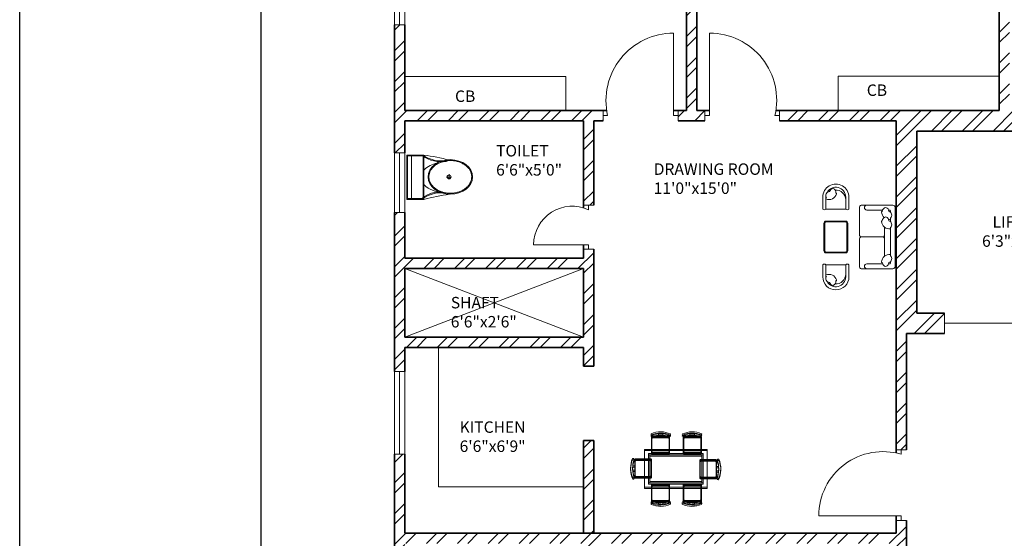
# Model space of a CAD drawing. Units: inches. Extents: x 2168 to 3056, y 1130 to 2629.
# Tile 21 of 42: x 2168 to 2598, y 2079 to 2305. Entities that reach past the tile are written whole.
import ezdxf

# ---------------------------------------------------------------- set-up
doc = ezdxf.new("R2010")
doc.units = ezdxf.units.IN
for name, color, linetype, lineweight in [('A-ANNO-DIMS', 2, 'Continuous', 18), ('A-ANNO-TEXT', 7, 'Continuous', 18), ('A-ANNO-TTLB', 7, 'Continuous', 25), ('A-AREA-IDEN', 7, 'Continuous', 18), ('A-DOOR', 21, 'Continuous', 18), ('A-EQPM-ELEV', 7, 'Continuous', 18), ('A-FLOR-CASE', 71, 'Continuous', 18), ('A-FLOR-FIXT', 9, 'Continuous', 18), ('A-FLOR-OTLN', 7, 'Continuous', 18), ('A-FURN', 8, 'Continuous', 13), ('A-GLAZ', 201, 'Continuous', 18), ('A-WALL', 7, 'Continuous', 35)]:
    doc.layers.add(name, color=color, linetype=linetype, lineweight=lineweight)
doc.layers.add('A-WALL-PATT', color=143, linetype='Continuous', lineweight=13, true_color=0x7aafdf)
doc.styles.get("Standard").update_dxf_attribs({"font": 'arial.ttf'})
doc.dimstyles.get("Standard").update_dxf_attribs({"dimtxt": 0.18, "dimasz": 0.18, "dimexe": 0.18, "dimexo": 0.0625, "dimgap": 0.09, "dimtad": 0, "dimtih": 1, "dimtoh": 1, "dimdec": 4, "dimzin": 0, "dimdsep": 46, "dimtxsty": 'Standard', "dimcen": 0.09, "dimadec": 0, "dimazin": 0, "dimtfac": 1, "dimtdec": 4, "dimtofl": 0, "dimtmove": 0, "dimatfit": 3, "dimfxl": 1, "dimtolj": 1, "dimtzin": 0, "dimarcsym": 0})

# ---------------------------------------------------------------- blocks, each defined once
blk = doc.blocks.new('A$C31115884')
for p, q in [((283, 498), (223, 498)), ((258, 466), (258, 523)), ((0, 200), (0, 0)), ((520, 200), (0, 200)), ((10, 190), (10, 10)), ((510, 190), (10, 190)), ((510, 10), (510, 190)), ((520, 0), (520, 200)), ((510, 54), (0, 54)), ((10, 10), (510, 10)), ((0, 0), (520, 0))]:
    blk.add_line(p, q)
blk.add_circle((256, 496), 23.6)
for centre, radius, start, end in [((2778, -205), 2807, 165.4549, 171.7133), ((-295, 403), 365, 324.2091, 9.3499), ((-295, 403), 375, 324.2091, 9.3499), ((806, 403), 365, 170.6501, 215.7909), ((3237, 905), 2807, 188.2867, 194.5451), ((384, 406), 293, 190.2774, 224.1564), ((139, 406), 293, 315.8436, 2.6563), ((806, 403), 375, 179.2036, 215.7909)]:
    blk.add_arc(centre, radius, start, end)
blk.add_ellipse((256, 510), major_axis=(0, -261), ratio=0.772727)
blk.add_open_spline([(256, 259), (263, 259), (270, 260), (288, 262), (299, 265), (320, 273), (330, 278), (350, 291), (360, 299), (378, 316), (386, 326), (402, 347), (409, 358), (421, 383), (427, 395), (436, 422), (440, 436), (445, 465), (447, 480), (448, 509), (448, 524), (445, 553), (443, 568), (436, 596), (432, 610), (422, 636), (416, 649), (402, 672), (395, 683), (379, 703), (370, 712), (351, 728), (341, 735), (321, 746), (310, 751), (289, 757), (278, 759), (256, 761), (245, 761), (223, 757), (212, 754), (191, 746), (181, 741), (161, 728), (151, 720), (133, 703), (125, 693), (110, 672), (103, 660), (90, 636), (85, 623), (76, 596), (72, 582), (67, 553), (66, 538), (64, 509), (65, 494), (68, 465), (70, 450), (77, 422), (81, 408), (91, 382), (97, 370), (111, 346), (118, 335), (135, 316), (144, 307), (162, 291), (172, 284), (193, 273), (203, 269), (225, 262), (236, 260), (250, 259), (253, 259), (256, 259)], degree=3, knots=[0, 0, 0, 0, 0.110105, 0.110105, 0.285049, 0.285049, 0.459994, 0.459994, 0.634938, 0.634938, 0.809882, 0.809882, 0.984827, 0.984827, 1.159771, 1.159771, 1.334715, 1.334715, 1.50966, 1.50966, 1.684604, 1.684604, 1.859549, 1.859549, 2.034493, 2.034493, 2.209437, 2.209437, 2.384382, 2.384382, 2.559326, 2.559326, 2.73427, 2.73427, 2.909215, 2.909215, 3.084159, 3.084159, 3.259103, 3.259103, 3.434048, 3.434048, 3.608992, 3.608992, 3.783936, 3.783936, 3.958881, 3.958881, 4.133825, 4.133825, 4.30877, 4.30877, 4.483714, 4.483714, 4.658658, 4.658658, 4.833603, 4.833603, 5.008547, 5.008547, 5.183491, 5.183491, 5.358436, 5.358436, 5.53338, 5.53338, 5.708324, 5.708324, 5.883269, 5.883269, 6.058213, 6.058213, 6.233158, 6.233158, 6.283185, 6.283185, 6.283185, 6.283185])
blk = doc.blocks.new('A$C1352')
at = {"color": 0}
for points in [[(0.003, 0.053), (0.003, 0.553, -0.414214), (0.053, 0.603), (0.753, 0.603, -0.414214), (0.803, 0.553), (0.803, 0.053, -0.414214), (0.753, 0.003), (0.053, 0.003, -0.414214)], [(0.023, 0.053), (0.023, 0.553, -0.414214), (0.053, 0.583), (0.753, 0.583, -0.414214), (0.783, 0.553), (0.783, 0.053, -0.414214), (0.753, 0.023), (0.053, 0.023, -0.414214)]]:
    blk.add_lwpolyline(points, format="xyb", close=True, dxfattribs=at)
blk = doc.blocks.new('CHAIR-LOUNGE')
blk.add_line((10.04, 5.71), (10.04, 10.98))
at = {"ltscale": 0.03}
blk.add_lwpolyline([(10.04, 10.98, -0.369229), (11.42, 10.98), (11.42, 5.7, -1), (0, 5.72), (0, 10.99, -0.369229), (1.39, 10.99)], format="xyb", close=True, dxfattribs=at)
blk.add_lwpolyline([(9.55, 3.71, -0.785087), (1.38, 5.71), (1.39, 10.99)], format="xyb")
for centre, radius, start, end in [((5.71, 6.93), 4.33, 179.9461, 273.658), ((5.63, 4.23), 0.207, 150.6238, 293.7423), ((8.67, 3.43), 3.35, 67.0143, 164.2857), ((8.41, 5.02), 1.73, 272.9922, 34.1401), ((5.71, 5.71), 4.33, 358.8536, 359.9461), ((7.44, 3.63), 1.78, 166.6403, 249.4695), ((6.65, 3.91), 1.95, 274.9999, 341.3534)]:
    blk.add_arc(centre, radius, start, end)
blk = doc.blocks.new('TABLE-DINING')
for points in [[(0, 17.02), (27.45, 17.02), (27.45, 0.55), (0, 0.55)], [(0, 17.02), (27.45, 17.02), (27.45, 0.55), (0, 0.55)], [(0, 16.47), (27.45, 16.47), (27.45, 0), (0, 0)], [(0, 16.47), (27.45, 16.47), (27.45, 0), (0, 0)], [(1.83, 15.19), (25.62, 15.19), (25.62, 2.38), (1.83, 2.38)], [(1.83, 15.19), (25.62, 15.19), (25.62, 2.38), (1.83, 2.38)], [(1.83, 14.64), (25.62, 14.64), (25.62, 1.83), (1.83, 1.83)], [(1.83, 14.64), (25.62, 14.64), (25.62, 1.83), (1.83, 1.83)], [(2.38, 14.64), (25.07, 14.64), (25.07, 2.93), (2.38, 2.93)], [(2.38, 14.64), (25.07, 14.64), (25.07, 2.93), (2.38, 2.93)], [(2.38, 14.09), (25.07, 14.09), (25.07, 2.38), (2.38, 2.38)], [(2.38, 14.09), (25.07, 14.09), (25.07, 2.38), (2.38, 2.38)]]:
    blk.add_lwpolyline(points, close=True)
blk = doc.blocks.new('CUPBOARD-BEDROOM')
blk.add_lwpolyline([(0, 14.89), (70.36, 14.89), (70.36, 0), (0, 0)], close=True)
blk = doc.blocks.new('CHAIR-DINING-SIDE')
for points in [[(7.85, 2.38, 0.414214), (8.33, 2.86), (8.33, 9.24, 0.414214), (7.85, 9.73), (0.91, 9.73, 0.414214), (0.42, 9.24), (0.42, 2.86, 0.414214), (0.91, 2.38), (7.85, 2.38)], [(7.85, 2.38, 0.414214), (8.33, 2.86), (8.33, 9.24, 0.414214), (7.85, 9.73), (0.91, 9.73, 0.414214), (0.42, 9.24), (0.42, 2.86, 0.414214), (0.91, 2.38), (7.85, 2.38)], [(7.85, 1.83, 0.414214), (8.33, 2.31), (8.33, 8.69, 0.414214), (7.85, 9.18), (0.91, 9.18, 0.414214), (0.42, 8.69), (0.42, 2.31, 0.414214), (0.91, 1.83), (7.85, 1.83)], [(7.85, 1.83, 0.414214), (8.33, 2.31), (8.33, 8.69, 0.414214), (7.85, 9.18), (0.91, 9.18, 0.414214), (0.42, 8.69), (0.42, 2.31, 0.414214), (0.91, 1.83), (7.85, 1.83)], [(8.06, 2.08, -0.175809), (0.59, 2.13, 0.578392), (0.02, 1.51, 0.214524), (8.46, 1.4, 0.552014), (8.06, 2.08, -0.065079)], [(8.06, 2.08, -0.175809), (0.59, 2.13, 0.578392), (0.02, 1.51, 0.214524), (8.46, 1.4, 0.552014), (8.06, 2.08, -0.065079)], [(8.06, 1.53, -0.175809), (0.59, 1.58, 0.578392), (0.02, 0.96, 0.214524), (8.46, 0.85, 0.552014), (8.06, 1.53, -0.065079)], [(8.06, 1.53, -0.175809), (0.59, 1.58, 0.578392), (0.02, 0.96, 0.214524), (8.46, 0.85, 0.552014), (8.06, 1.53, -0.065079)], [(3.34, 2.38), (3.34, 1.5, -0.064759)], [(3.34, 2.38), (3.34, 1.5, -0.064759)], [(3.34, 1.83), (3.34, 0.95, -0.064759)], [(3.34, 1.83), (3.34, 0.95, -0.064759)]]:
    blk.add_lwpolyline(points, format="xyb")
for points in [[(7.84, 2.6), (1.13, 2.6, -0.414214), (0.64, 3.08), (0.64, 9.02, -0.414214), (1.13, 9.51), (7.84, 9.51, -0.512069), (8.11, 9.02), (8.11, 3.08, -0.512069)], [(7.84, 2.6), (1.13, 2.6, -0.414214), (0.64, 3.08), (0.64, 9.02, -0.414214), (1.13, 9.51), (7.84, 9.51, -0.512069), (8.11, 9.02), (8.11, 3.08, -0.512069)], [(7.84, 2.05), (1.13, 2.05, -0.414214), (0.64, 2.53), (0.64, 8.48, -0.414214), (1.13, 8.96), (7.84, 8.96, -0.512069), (8.11, 8.48), (8.11, 2.53, -0.512069)], [(7.84, 2.05), (1.13, 2.05, -0.414214), (0.64, 2.53), (0.64, 8.48, -0.414214), (1.13, 8.96), (7.84, 8.96, -0.512069), (8.11, 8.48), (8.11, 2.53, -0.512069)]]:
    blk.add_lwpolyline(points, format="xyb", close=True)
for points in [[(5.29, 1.48), (5.29, 2.38)], [(5.29, 1.48), (5.29, 2.38)], [(5.29, 0.93), (5.29, 1.83)], [(5.29, 0.93), (5.29, 1.83)]]:
    blk.add_lwpolyline(points)
blk = doc.blocks.new('WIN-60-OPPOSED-JAMBS')
for p, q in [((2.25, 60), (0, 60)), ((0, 60), (4.5, 60)), ((0, 60), (0, 0)), ((2.25, 0), (2.25, 60)), ((4.5, 60), (4.5, 0)), ((0, 0), (4.5, 0)), ((4.5, 0), (2.25, 0))]:
    blk.add_line(p, q)
blk = doc.blocks.new('WIN-36')
for p, q in [((2.25, 36), (0, 36)), ((0, 36), (4.5, 36)), ((0, 36), (0, 0)), ((2.25, 0), (2.25, 36)), ((4.5, 36), (4.5, 0)), ((0, 0), (4.5, 0)), ((4.5, 0), (2.25, 0))]:
    blk.add_line(p, q)
blk = doc.blocks.new('*D41')
at = {"layer": 'A-ANNO-DIMS', "color": 0, "lineweight": -2, "transparency": 16777216}
for p, q in [((2331.73, 2478.39), (2273.32, 2478.39)), ((2273.5, 2478.21), (2273.5, 1928.07)), ((2273.5, 1377.57), (2273.5, 1927.71)), ((2331.73, 1377.39), (2273.32, 1377.39))]:
    blk.add_line(p, q, dxfattribs=at)
at = {"layer": 'A-ANNO-DIMS', "color": 0, "transparency": 16777216}
for points in [[(2273.47, 2478.21), (2273.53, 2478.21), (2273.5, 2478.39)], [(2273.47, 1377.57), (2273.53, 1377.57), (2273.5, 1377.39)]]:
    blk.add_solid(points, dxfattribs=at)
at = {"layer": 'Defpoints', "color": 0, "transparency": 16777216}
for p in [(2273.5, 2478.39), (2331.8, 2478.39), (2331.8, 1377.39)]:
    blk.add_point(p, dxfattribs=at)
at = {"layer": 'A-ANNO-DIMS', "color": 0, "transparency": 16777216, "insert": (2273.5, 1927.89), "char_height": 0.18, "attachment_point": 5}
blk.add_mtext('\\A1;1101', dxfattribs=at)

msp = doc.modelspace()

# ---------------------------------------------------------------- hatches: boundary and pattern name
at = {"layer": 'A-WALL-PATT'}
h = msp.add_hatch(dxfattribs=at)
h.set_pattern_fill('ANSI32', color=256)
h.paths.add_polyline_path([(2463.8, 2409.39), (2467.39, 2409.39), (2467.39, 2413.89), (2454.77, 2413.89), (2454.77, 2411.64), (2454.77, 2409.39), (2459.3, 2409.39), (2459.3, 2265.39), (2455.64, 2265.39), (2455.64, 2260.89), (2467.35, 2260.89), (2467.35, 2263.14), (2467.35, 2265.39), (2463.8, 2265.39)])
h.paths.add_polyline_path([(2431.6, 2413.89), (2409.65, 2413.89), (2409.65, 2409.39), (2431.6, 2409.39), (2431.6, 2411.64)])
h.paths.add_polyline_path([(2349.65, 2413.89), (2331.8, 2413.89), (2331.8, 2362.67), (2336.3, 2362.67), (2336.3, 2409.39), (2349.65, 2409.39), (2349.65, 2411.64)])
h.paths.add_polyline_path([(2634.15, 2411.64), (2634.15, 2413.89), (2562.29, 2413.89), (2562.29, 2409.39), (2595.8, 2409.39), (2595.8, 2280.31), (2595.83, 2280.31), (2595.83, 2265.39), (2499.91, 2265.39), (2499.91, 2260.89), (2550.8, 2260.89), (2550.8, 2117.31), (2555.3, 2117.31), (2555.3, 2168.08), (2571.93, 2168.08), (2571.93, 2176.89), (2559.8, 2176.89), (2559.8, 2256.39), (2640.8, 2256.39), (2640.8, 2176.89), (2626.43, 2176.89), (2626.43, 2168.08), (2645.3, 2168.08), (2645.3, 2116.64), (2649.8, 2116.64), (2649.8, 2260.89), (2691.25, 2260.89), (2691.25, 2263.14), (2691.25, 2265.39), (2670.65, 2265.39), (2670.65, 2265.36), (2600.3, 2265.36), (2600.3, 2280.26), (2600.3, 2409.39), (2634.15, 2409.39)])
h.paths.add_polyline_path([(2600.3, 2473.89), (2612.84, 2473.89), (2612.84, 2478.39), (2572.64, 2478.39), (2572.64, 2473.89), (2595.8, 2473.89), (2595.8, 2413.89), (2600.3, 2413.89)])
h.paths.add_polyline_path([(2535.8, 2473.89), (2548.64, 2473.89), (2548.64, 2478.39), (2531.4, 2478.39), (2531.4, 2413.89), (2521.6, 2413.89), (2521.6, 2409.39), (2539.24, 2409.39), (2539.24, 2411.64), (2539.24, 2413.89), (2535.8, 2413.89)])
h.paths.add_polyline_path([(2664.8, 2478.39), (2636.84, 2478.39), (2636.84, 2473.89), (2660.3, 2473.89), (2660.3, 2413.89), (2656.17, 2413.89), (2656.17, 2409.39), (2671.68, 2409.39), (2671.68, 2411.64), (2671.68, 2413.89), (2664.8, 2413.89)])
h.paths.add_polyline_path([(2705.94, 2413.89), (2695.68, 2413.89), (2695.68, 2409.39), (2705.94, 2409.39)])
h.paths.add_polyline_path([(2741.35, 2413.89), (2728.73, 2413.89), (2728.73, 2411.64), (2728.73, 2409.39), (2732.3, 2409.39), (2732.3, 2265.39), (2725.73, 2265.39), (2725.73, 2260.89), (2740.92, 2260.89), (2740.92, 2263.14), (2740.92, 2265.39), (2736.8, 2265.39), (2736.8, 2409.39), (2741.35, 2409.39)])
h.paths.add_polyline_path([(2785.65, 2413.89), (2764.55, 2413.89), (2764.49, 2409.39), (2785.65, 2409.39), (2785.65, 2411.64)])
h.paths.add_polyline_path([(2864.3, 2413.89), (2845.65, 2413.89), (2845.65, 2409.39), (2859.8, 2409.39), (2859.8, 2368.43), (2864.3, 2368.43)])
h.paths.add_polyline_path([(2864.3, 2308.43), (2862.05, 2308.43), (2859.8, 2308.43), (2859.8, 2265.39), (2774.48, 2265.39), (2774.48, 2263.14), (2774.48, 2260.89), (2781.8, 2260.89), (2781.8, 2226.65), (2786.3, 2226.65), (2786.3, 2260.89), (2859.8, 2260.89), (2859.8, 2241.35), (2864.3, 2241.35)])
h.paths.add_polyline_path([(2864.3, 2217.35), (2862.05, 2217.35), (2859.8, 2217.35), (2859.8, 2200.89), (2786.3, 2200.89), (2786.3, 2205.93), (2784.05, 2205.93), (2781.8, 2205.93), (2781.8, 2150.97), (2786.3, 2150.97), (2786.3, 2161.89), (2859.8, 2161.89), (2859.8, 2144.42), (2864.3, 2144.42)])
h.paths.add_polyline_path([(2859.8, 2196.39), (2859.8, 2166.39), (2786.3, 2166.39), (2786.3, 2196.39)], flags=16)
h.paths.add_polyline_path([(2864.3, 2108.42), (2862.05, 2108.42), (2859.8, 2108.42), (2859.8, 2080.89), (2786.3, 2080.89), (2786.3, 2111.99), (2781.8, 2111.99), (2781.8, 2080.89), (2649.8, 2080.89), (2649.8, 2086.04), (2647.55, 2086.04), (2645.3, 2086.04), (2645.3, 2071.74), (2649.8, 2071.74), (2649.8, 2076.39), (2781.8, 2076.39), (2781.8, 2041.79), (2786.3, 2041.79), (2786.3, 2076.39), (2859.8, 2076.39), (2859.8, 2058.58), (2864.3, 2058.58)])
h.paths.add_polyline_path([(2864.3, 2022.58), (2859.8, 2022.58), (2859.8, 1992.39), (2786.3, 1992.39), (2786.3, 1999.57), (2781.8, 1999.57), (2781.8, 1848.09), (2784.05, 1848.09), (2786.3, 1848.09), (2786.3, 1851.39), (2859.8, 1851.39), (2859.8, 1838.26), (2864.3, 1838.26)], flags=17)
h.paths.add_polyline_path([(2859.8, 1987.89), (2859.8, 1855.89), (2786.3, 1855.89), (2786.3, 1987.89)], flags=16)
h.paths.add_polyline_path([(2823.05, 1987.89), (2841.42, 1921.89), (2823.05, 1855.89)], flags=0)
h.paths.add_polyline_path([(2864.3, 1814.26), (2859.8, 1814.26), (2859.8, 1791.39), (2786.3, 1791.39), (2786.3, 1825.66), (2784.05, 1825.66), (2781.8, 1825.66), (2781.8, 1791.39), (2720.15, 1791.39), (2720.15, 1791.27), (2649.8, 1791.27), (2649.8, 1806.16), (2649.8, 2038.98), (2647.55, 2038.98), (2645.3, 2038.98), (2645.3, 1783.93), (2649.8, 1783.93), (2649.8, 1786.89), (2781.8, 1786.89), (2781.8, 1746.79), (2786.3, 1746.79), (2786.3, 1786.89), (2859.8, 1786.89), (2859.8, 1770.08), (2864.3, 1770.08)])
h.paths.add_polyline_path([(2864.3, 1734.08), (2862.05, 1734.08), (2859.8, 1734.08), (2859.8, 1705.89), (2786.3, 1705.89), (2786.3, 1714.17), (2781.8, 1714.17), (2781.8, 1660.53), (2786.3, 1660.53), (2786.3, 1666.89), (2859.8, 1666.89), (2859.8, 1648.34), (2864.3, 1648.34)])
h.paths.add_polyline_path([(2786.3, 1701.39), (2859.8, 1701.39), (2859.8, 1671.39), (2786.3, 1671.39)], flags=16)
h.paths.add_polyline_path([(2649.8, 1756.58), (2647.55, 1756.58), (2645.3, 1756.58), (2645.3, 1606.89), (2555.3, 1606.89), (2555.3, 1749.51), (2553.05, 1749.51), (2550.8, 1749.51), (2550.8, 1606.89), (2503.01, 1606.89), (2503.01, 1604.64), (2503.01, 1602.39), (2595.8, 1602.39), (2595.85, 1602.39), (2595.85, 1587.5), (2595.8, 1458.39), (2561.5, 1458.39), (2561.5, 1456.14), (2561.5, 1453.89), (2595.8, 1453.89), (2595.8, 1381.89), (2573.44, 1381.89), (2573.44, 1377.39), (2613.01, 1377.39), (2613.01, 1379.64), (2613.01, 1381.89), (2600.3, 1381.89), (2600.3, 1453.89), (2634.33, 1453.89), (2634.33, 1458.39), (2600.3, 1458.39), (2600.3, 1602.39), (2670.65, 1602.39), (2694.09, 1602.39), (2694.09, 1606.89), (2649.8, 1606.89)])
h.paths.add_polyline_path([(2736.8, 1602.39), (2741.56, 1602.39), (2741.56, 1606.89), (2726.2, 1606.89), (2726.2, 1604.64), (2726.2, 1602.39), (2732.3, 1602.39), (2732.3, 1458.39), (2727.9, 1458.39), (2727.9, 1453.89), (2740.82, 1453.89), (2740.82, 1456.14), (2740.82, 1458.39), (2736.8, 1458.39)])
h.paths.add_polyline_path([(2859.8, 1606.89), (2786.3, 1606.89), (2786.3, 1637.33), (2784.05, 1637.33), (2781.8, 1637.33), (2781.8, 1606.89), (2775.61, 1606.89), (2775.61, 1602.39), (2859.8, 1602.39)])
h.paths.add_polyline_path([(2864.3, 1624.34), (2862.05, 1624.34), (2859.8, 1624.34), (2859.8, 1570.39), (2864.3, 1570.39)])
h.paths.add_polyline_path([(2864.3, 1510.39), (2862.05, 1510.39), (2859.8, 1510.39), (2859.8, 1458.39), (2846.73, 1458.39), (2846.73, 1456.14), (2846.73, 1453.89), (2864.3, 1453.89)])
h.paths.add_polyline_path([(2786.73, 1458.39), (2765.44, 1458.39), (2765.44, 1453.89), (2786.73, 1453.89)])
h.paths.add_polyline_path([(2706, 1458.39), (2695.36, 1458.39), (2695.36, 1453.89), (2706, 1453.89), (2706, 1456.14)])
h.paths.add_polyline_path([(2671.36, 1456.14), (2671.36, 1458.39), (2655.99, 1458.39), (2655.99, 1456.14), (2655.99, 1453.89), (2660.3, 1453.89), (2660.3, 1381.89), (2637.01, 1381.89), (2637.01, 1377.39), (2664.8, 1377.39), (2664.8, 1453.89), (2671.36, 1453.89)], flags=17)
h.paths.add_polyline_path([(2539.83, 1458.39), (2520.24, 1458.39), (2520.24, 1453.89), (2531.3, 1453.89), (2531.3, 1377.39), (2546.45, 1377.39), (2546.45, 1379.64), (2546.45, 1381.89), (2535.8, 1381.89), (2535.8, 1453.89), (2539.83, 1453.89)], flags=17)
h.paths.add_polyline_path([(2496.24, 1458.39), (2489.13, 1458.39), (2489.13, 1453.89), (2496.24, 1453.89), (2496.24, 1456.14)])
h.paths.add_polyline_path([(2467.43, 1456.14), (2467.43, 1458.39), (2463.8, 1458.39), (2463.8, 1602.39), (2468.24, 1602.39), (2468.24, 1605.7), (2468.24, 1606.89), (2454.6, 1606.89), (2454.6, 1602.39), (2459.3, 1602.39), (2459.3, 1458.39), (2454.24, 1458.39), (2454.24, 1453.89), (2467.43, 1453.89)])
h.paths.add_polyline_path([(2431.6, 1456.14), (2431.6, 1458.39), (2411.39, 1458.39), (2411.39, 1453.89), (2431.6, 1453.89)])
h.paths.add_polyline_path([(2351.39, 1458.39), (2336.3, 1458.39), (2336.3, 1490.69), (2334.05, 1490.69), (2331.8, 1490.69), (2331.8, 1453.89), (2351.39, 1453.89), (2351.39, 1456.14)])
h.paths.add_polyline_path([(2336.3, 1629.7), (2331.8, 1629.7), (2331.8, 1552.32), (2336.3, 1552.32), (2336.3, 1602.39), (2406.65, 1602.39), (2423.47, 1602.39), (2423.47, 1606.89), (2418.8, 1606.89), (2418.8, 1643.68), (2416.55, 1643.68), (2414.3, 1643.68), (2414.3, 1606.89), (2336.3, 1606.89)])
h.paths.add_polyline_path([(2418.8, 1714.38), (2414.3, 1714.38), (2414.3, 1705.89), (2336.3, 1705.89), (2336.3, 1731.32), (2334.05, 1731.32), (2331.8, 1731.32), (2331.8, 1653.7), (2334.05, 1653.7), (2336.3, 1653.7), (2336.3, 1666.89), (2414.3, 1666.89), (2414.3, 1663.59), (2418.8, 1663.59)])
h.paths.add_polyline_path([(2336.3, 1701.39), (2414.3, 1701.39), (2414.3, 1671.39), (2336.3, 1671.39)], flags=16)
h.paths.add_polyline_path([(2555.3, 2040.06), (2550.8, 2040.06), (2550.8, 1791.39), (2550.56, 1791.2), (2480.2, 1791.2), (2418.8, 1791.39), (2418.8, 1825.45), (2416.55, 1825.45), (2414.3, 1825.45), (2414.3, 1791.39), (2336.3, 1791.39), (2336.3, 1806.41), (2331.8, 1806.41), (2331.8, 1767.32), (2336.3, 1767.32), (2336.3, 1786.89), (2414.3, 1786.89), (2414.3, 1745.46), (2418.8, 1745.46), (2418.8, 1786.89), (2550.8, 1786.89), (2550.8, 1783.01), (2555.3, 1783.01)])
h.paths.add_polyline_path([(2418.8, 1923.39), (2423.21, 1923.39), (2423.21, 1925.64), (2423.21, 1927.89), (2418.8, 1927.89), (2418.8, 2000.05), (2414.3, 2000.05), (2414.3, 1992.39), (2336.3, 1992.39), (2336.3, 1987.89), (2414.3, 1987.89), (2414.3, 1855.89), (2336.3, 1855.89), (2336.3, 1851.39), (2414.3, 1851.39), (2414.3, 1846.76), (2418.8, 1846.76)], flags=17)
h.paths.add_polyline_path([(2336.3, 2019.29), (2334.05, 2019.29), (2331.8, 2019.29), (2331.8, 1830.41), (2336.3, 1830.41)], flags=17)
h.paths.add_polyline_path([(2550.8, 1927.89), (2453.54, 1927.89), (2453.54, 1925.64), (2453.54, 1923.39), (2550.8, 1923.39)], flags=17)
h.paths.add_polyline_path([(2744.99, 1927.89), (2649.8, 1927.89), (2649.8, 1923.39), (2744.99, 1923.39), (2744.99, 1925.64)], flags=17)
h.paths.add_polyline_path([(2555.3, 2086.46), (2553.05, 2086.46), (2550.8, 2086.46), (2550.8, 2080.89), (2418.8, 2080.89), (2336.3, 2080.89), (2336.3, 2115.4), (2334.05, 2115.4), (2331.8, 2115.4), (2331.8, 2055.29), (2336.3, 2055.29), (2336.3, 2076.39), (2550.8, 2076.39), (2550.8, 2071.54), (2555.3, 2071.54)])
h.paths.add_polyline_path([(2418.8, 2121.39), (2414.3, 2121.39), (2414.3, 2080.89), (2418.8, 2080.89)])
h.paths.add_polyline_path([(2418.8, 2076.39), (2414.3, 2076.39), (2414.3, 2035.12), (2418.8, 2035.12)])
h.paths.add_polyline_path([(2422.87, 2263.14), (2422.87, 2265.39), (2406.65, 2265.39), (2406.65, 2265.36), (2336.3, 2265.36), (2336.3, 2280.25), (2336.3, 2302.67), (2334.05, 2302.67), (2331.8, 2302.67), (2331.8, 2246.85), (2336.3, 2246.85), (2336.3, 2260.89), (2414.3, 2260.89), (2414.3, 2224), (2418.8, 2224), (2418.8, 2260.89), (2422.87, 2260.89)])
h.paths.add_polyline_path([(2418.8, 2204.78), (2416.55, 2204.78), (2414.3, 2204.78), (2414.3, 2200.89), (2336.3, 2200.89), (2336.3, 2220.85), (2331.8, 2220.85), (2331.8, 2151.4), (2336.3, 2151.4), (2336.3, 2161.89), (2414.3, 2161.89), (2414.3, 2153.73), (2418.8, 2153.73)])
h.paths.add_polyline_path([(2414.3, 2196.39), (2414.3, 2166.39), (2336.3, 2166.39), (2336.3, 2196.39)], flags=16)
h.paths.add_polyline_path([(2375.3, 2181.39), (2336.3, 2166.39), (2336.3, 2196.39)], flags=0)
h.paths.add_polyline_path([(2809.6, 2172.34), (2838.8, 2172.34), (2838.8, 2191), (2809.6, 2191)], flags=8)
h.paths.add_polyline_path([(2849.75, 1919.59), (2849.75, 1952.67), (2831.09, 1952.67), (2831.09, 1919.59)], flags=8)
h.paths.add_polyline_path([(2808.87, 1901.97), (2808.87, 1937.85), (2790.15, 1937.85), (2790.15, 1901.97)], flags=8)
h.paths.add_polyline_path([(2806.28, 1671.9), (2835.49, 1671.9), (2835.49, 1690.55), (2806.28, 1690.55)], flags=8)
h.paths.add_polyline_path([(2353.19, 1676.55), (2382.39, 1676.55), (2382.39, 1695.21), (2353.19, 1695.21)], flags=8)
h.paths.add_polyline_path([(2360.08, 1832.31), (2389.24, 1832.31), (2389.24, 1850.97), (2360.08, 1850.97)], flags=25)
h.paths.add_polyline_path([(2354.82, 2167.82), (2384.03, 2167.82), (2384.03, 2186.48), (2354.82, 2186.48)], flags=8)

# ---------------------------------------------------------------- linework, layer by layer
at = {"layer": 'A-ANNO-TTLB'}
msp.add_lwpolyline([(2168.16, 2629.19), (3055.63, 2629.19), (3055.63, 1130.19), (2168.16, 1130.19)], close=True, dxfattribs=at)
at = {"layer": 'A-DOOR'}
for p, q in [((2453.64, 2263.16), (2453.64, 2299.16)), ((2469.35, 2263.14), (2469.35, 2299.14)), ((2422.87, 2265.39), (2422.87, 2260.89)), ((2422.87, 2260.89), (2422.87, 2263.14)), ((2422.87, 2263.14), (2424.87, 2263.14)), ((2455.64, 2263.14), (2453.64, 2263.16)), ((2455.64, 2265.39), (2455.64, 2260.89)), ((2455.64, 2260.89), (2455.64, 2263.14)), ((2467.35, 2265.39), (2467.35, 2260.89)), ((2467.35, 2260.89), (2467.35, 2263.14)), ((2467.35, 2263.14), (2469.35, 2263.14)), ((2499.91, 2263.14), (2497.91, 2263.14)), ((2499.91, 2265.39), (2499.91, 2260.89)), ((2499.91, 2260.89), (2499.91, 2265.39)), ((2414.3, 2224), (2418.8, 2224)), ((2418.8, 2224), (2416.55, 2224)), ((2416.55, 2224), (2416.55, 2222)), ((2416.55, 2206.78), (2392.55, 2206.78)), ((2416.55, 2204.78), (2416.55, 2206.78)), ((2414.3, 2204.78), (2418.8, 2204.78)), ((2418.8, 2204.78), (2416.55, 2204.78)), ((2550.8, 2117.31), (2555.3, 2117.31)), ((2553.05, 2117.31), (2553.05, 2115.31)), ((2553.05, 2088.46), (2517.05, 2088.46)), ((2550.8, 2086.46), (2555.3, 2086.46)), ((2553.05, 2086.46), (2553.05, 2088.46)), ((2555.3, 2086.46), (2553.05, 2086.46))]:
    msp.add_line(p, q, dxfattribs=at)
for centre, radius, start, end in [((2453.64, 2269.65), 29.5, 90, 192.7563), ((2469.35, 2269.81), 29.33, 346.8551, 90), ((2409.37, 2206.78), 16.82, 64.7394, 180), ((2545.06, 2088.46), 28.01, 73.4344, 180)]:
    msp.add_arc(centre, radius, start, end, dxfattribs=at)
at = {"layer": 'A-EQPM-ELEV'}
for p, q in [((2571.93, 2176.89), (2571.93, 2168.08)), ((2626.43, 2172.48), (2571.93, 2172.48))]:
    msp.add_line(p, q, dxfattribs=at)
at = {"layer": 'A-FLOR-CASE'}
for p, q in [((2350.95, 2101.14), (2350.95, 2161.89)), ((2414.3, 2101.14), (2350.95, 2101.14))]:
    msp.add_line(p, q, dxfattribs=at)
at = {"layer": 'A-FLOR-OTLN'}
for p, q in [((2336.3, 2166.39), (2414.3, 2196.39)), ((2336.3, 2196.39), (2414.3, 2166.39)), ((2414.3, 2166.39), (2414.3, 2166.39))]:
    msp.add_line(p, q, dxfattribs=at)
at = {"layer": 'A-FURN'}
for p, q in [((2544.93, 2221.92), (2538, 2221.92)), ((2547.56, 2221.92), (2548.04, 2221.92)), ((2548.38, 2221.57), (2548.38, 2220.94)), ((2548.38, 2216.78), (2548.38, 2218.44)), ((2548.38, 2217.42), (2548.38, 2216.78)), ((2548.38, 2201.87), (2548.38, 2214.29)), ((2538, 2198.39), (2544.93, 2198.39)), ((2547.56, 2198.39), (2548.04, 2198.39)), ((2548.38, 2198.74), (2548.38, 2199.37))]:
    msp.add_line(p, q, dxfattribs=at)
at = {"layer": 'A-FURN', "ltscale": 0.03}
msp.add_lwpolyline([(2535.58, 2210.15, 0.414214), (2534.89, 2209.45), (2534.89, 2197.01, 0.414214), (2535.58, 2196.31), (2549.42, 2196.31, 0.414214), (2550.46, 2197.35), (2550.46, 2222.96, 0.414214), (2549.42, 2224), (2535.58, 2224, 0.414214), (2534.89, 2223.3), (2534.89, 2210.86, 0.414214), (2535.58, 2210.16)], format="xyb", dxfattribs=at)
at = {"layer": 'A-FURN'}
for points in [[(2545.7, 2214.42), (2545.7, 2211.02, -0.414214), (2544.84, 2210.16), (2535.75, 2210.16, -0.414214), (2534.89, 2211.02), (2534.89, 2223.13, -0.414214), (2535.75, 2224)], [(2545.7, 2202.32), (2545.7, 2209.29, 0.414214), (2544.84, 2210.16), (2535.75, 2210.16, 0.414214), (2534.89, 2209.29), (2534.89, 2197.18, 0.414214), (2535.75, 2196.31)], [(2444.28, 2123.6, -0.175809), (2451.76, 2123.55, 0.578392), (2452.32, 2124.17, 0.214524), (2443.89, 2124.28, 0.552014), (2444.28, 2123.6, -0.065079)], [(2444.28, 2123.6, -0.175809), (2451.76, 2123.55, 0.578392), (2452.32, 2124.17, 0.214524), (2443.89, 2124.28, 0.552014), (2444.28, 2123.6, -0.065079)], [(2444.28, 2123.05, -0.175809), (2451.76, 2123, 0.578392), (2452.32, 2123.62, 0.214524), (2443.89, 2123.73, 0.552014), (2444.28, 2123.05, -0.065079)], [(2444.28, 2123.05, -0.175809), (2451.76, 2123, 0.578392), (2452.32, 2123.62, 0.214524), (2443.89, 2123.73, 0.552014), (2444.28, 2123.05, -0.065079)], [(2449, 2123.3), (2449, 2124.18, -0.064759)], [(2449, 2123.3), (2449, 2124.18, -0.064759)], [(2458.05, 2123.55, -0.578392), (2457.49, 2124.17, -0.214524), (2465.92, 2124.28, -0.552014), (2465.53, 2123.6, 0.175809), (2458.05, 2123.55)], [(2458.05, 2123.55, -0.578392), (2457.49, 2124.17, -0.214524), (2465.92, 2124.28, -0.552014), (2465.53, 2123.6, 0.175809), (2458.05, 2123.55)], [(2458.05, 2123, -0.578392), (2457.49, 2123.62, -0.214524), (2465.92, 2123.73, -0.552014), (2465.53, 2123.05, 0.175809), (2458.05, 2123)], [(2458.05, 2123, -0.578392), (2457.49, 2123.62, -0.214524), (2465.92, 2123.73, -0.552014), (2465.53, 2123.05, 0.175809), (2458.05, 2123)], [(2460.81, 2123.3), (2460.81, 2124.18, 0.064759)], [(2460.81, 2123.3), (2460.81, 2124.18, 0.064759)], [(2451.44, 2123.3), (2444.5, 2123.3, 0.414214), (2444.02, 2122.82), (2444.02, 2116.44, 0.414214), (2444.5, 2115.95), (2451.44, 2115.95, 0.414214), (2451.93, 2116.44), (2451.93, 2122.82, 0.414214), (2451.44, 2123.3)], [(2451.44, 2123.3), (2444.5, 2123.3, 0.414214), (2444.02, 2122.82), (2444.02, 2116.44, 0.414214), (2444.5, 2115.95), (2451.44, 2115.95, 0.414214), (2451.93, 2116.44), (2451.93, 2122.82, 0.414214), (2451.44, 2123.3)], [(2451.44, 2122.75), (2444.5, 2122.75, 0.414214), (2444.02, 2122.27), (2444.02, 2115.89, 0.414214), (2444.5, 2115.4), (2451.44, 2115.4, 0.414214), (2451.93, 2115.89), (2451.93, 2122.27, 0.414214), (2451.44, 2122.75)], [(2451.44, 2122.75), (2444.5, 2122.75, 0.414214), (2444.02, 2122.27), (2444.02, 2115.89, 0.414214), (2444.5, 2115.4), (2451.44, 2115.4, 0.414214), (2451.93, 2115.89), (2451.93, 2122.27, 0.414214), (2451.44, 2122.75)], [(2449, 2122.75), (2449, 2123.63, -0.064759)], [(2449, 2122.75), (2449, 2123.63, -0.064759)], [(2465.31, 2123.3, -0.414214), (2465.79, 2122.82), (2465.79, 2116.44, -0.414214), (2465.31, 2115.95), (2458.37, 2115.95, -0.414214), (2457.88, 2116.44), (2457.88, 2122.82, -0.414214), (2458.37, 2123.3), (2465.31, 2123.3)], [(2465.31, 2123.3, -0.414214), (2465.79, 2122.82), (2465.79, 2116.44, -0.414214), (2465.31, 2115.95), (2458.37, 2115.95, -0.414214), (2457.88, 2116.44), (2457.88, 2122.82, -0.414214), (2458.37, 2123.3), (2465.31, 2123.3)], [(2465.31, 2122.75, -0.414214), (2465.79, 2122.27), (2465.79, 2115.89, -0.414214), (2465.31, 2115.4), (2458.37, 2115.4, -0.414214), (2457.88, 2115.89), (2457.88, 2122.27, -0.414214), (2458.37, 2122.75), (2465.31, 2122.75)], [(2465.31, 2122.75, -0.414214), (2465.79, 2122.27), (2465.79, 2115.89, -0.414214), (2465.31, 2115.4), (2458.37, 2115.4, -0.414214), (2457.88, 2115.89), (2457.88, 2122.27, -0.414214), (2458.37, 2122.75), (2465.31, 2122.75)], [(2460.81, 2122.75), (2460.81, 2123.63, 0.064759)], [(2460.81, 2122.75), (2460.81, 2123.63, 0.064759)], [(2436.46, 2105.55, -0.578392), (2435.84, 2104.98, -0.214524), (2435.73, 2113.42, -0.552014), (2436.41, 2113.03, 0.175809), (2436.46, 2105.55)], [(2436.46, 2105.55, -0.578392), (2435.84, 2104.98, -0.214524), (2435.73, 2113.42, -0.552014), (2436.41, 2113.03, 0.175809), (2436.46, 2105.55)], [(2436.46, 2105, -0.578392), (2435.84, 2104.44, -0.214524), (2435.73, 2112.87, -0.552014), (2436.41, 2112.48, 0.175809), (2436.46, 2105)], [(2436.46, 2105, -0.578392), (2435.84, 2104.44, -0.214524), (2435.73, 2112.87, -0.552014), (2436.41, 2112.48, 0.175809), (2436.46, 2105)], [(2436.71, 2112.81, -0.414214), (2437.19, 2113.29), (2443.57, 2113.29, -0.414214), (2444.06, 2112.81), (2444.06, 2105.87, -0.414214), (2443.57, 2105.38), (2437.19, 2105.38, -0.414214), (2436.71, 2105.87), (2436.71, 2112.81)], [(2436.71, 2112.81, -0.414214), (2437.19, 2113.29), (2443.57, 2113.29, -0.414214), (2444.06, 2112.81), (2444.06, 2105.87, -0.414214), (2443.57, 2105.38), (2437.19, 2105.38, -0.414214), (2436.71, 2105.87), (2436.71, 2112.81)], [(2436.71, 2112.26, -0.414214), (2437.19, 2112.75), (2443.57, 2112.75, -0.414214), (2444.06, 2112.26), (2444.06, 2105.32, -0.414214), (2443.57, 2104.83), (2437.19, 2104.83, -0.414214), (2436.71, 2105.32), (2436.71, 2112.26)], [(2436.71, 2112.26, -0.414214), (2437.19, 2112.74), (2443.57, 2112.74, -0.414214), (2444.06, 2112.26), (2444.06, 2105.32, -0.414214), (2443.57, 2104.83), (2437.19, 2104.83, -0.414214), (2436.71, 2105.32), (2436.71, 2112.26)], [(2472.44, 2112.57, 0.414214), (2471.96, 2113.06), (2465.58, 2113.06, 0.414214), (2465.09, 2112.57), (2465.09, 2105.63, 0.414214), (2465.58, 2105.15), (2471.96, 2105.15, 0.414214), (2472.44, 2105.63), (2472.44, 2112.57)], [(2472.44, 2112.57, 0.414214), (2471.96, 2113.06), (2465.58, 2113.06, 0.414214), (2465.09, 2112.57), (2465.09, 2105.63, 0.414214), (2465.58, 2105.14), (2471.96, 2105.14, 0.414214), (2472.44, 2105.63), (2472.44, 2112.57)], [(2472.44, 2112.02, 0.414214), (2471.96, 2112.51), (2465.58, 2112.51, 0.414214), (2465.09, 2112.02), (2465.09, 2105.08, 0.414214), (2465.58, 2104.6), (2471.96, 2104.6, 0.414214), (2472.44, 2105.08), (2472.44, 2112.02)], [(2472.44, 2112.02, 0.414214), (2471.96, 2112.51), (2465.58, 2112.51, 0.414214), (2465.09, 2112.02), (2465.09, 2105.08, 0.414214), (2465.58, 2104.6), (2471.96, 2104.6, 0.414214), (2472.44, 2105.08), (2472.44, 2112.02)], [(2472.74, 2112.79, -0.175809), (2472.69, 2105.31, 0.578392), (2473.31, 2104.75, 0.214524), (2473.42, 2113.19, 0.552014), (2472.74, 2112.79, -0.065079)], [(2472.74, 2112.79, -0.175809), (2472.69, 2105.31, 0.578392), (2473.31, 2104.75, 0.214524), (2473.42, 2113.19, 0.552014), (2472.74, 2112.79, -0.065079)], [(2472.74, 2112.24, -0.175809), (2472.69, 2104.76, 0.578392), (2473.31, 2104.2, 0.214524), (2473.42, 2112.64, 0.552014), (2472.74, 2112.24, -0.065079)], [(2472.74, 2112.24, -0.175809), (2472.69, 2104.76, 0.578392), (2473.31, 2104.2, 0.214524), (2473.42, 2112.64, 0.552014), (2472.74, 2112.24, -0.065079)], [(2436.71, 2108.31), (2435.83, 2108.31, 0.064759)], [(2436.71, 2108.31), (2435.83, 2108.31, 0.064759)], [(2436.71, 2107.76), (2435.83, 2107.76, 0.064759)], [(2436.71, 2107.76), (2435.83, 2107.76, 0.064759)], [(2472.44, 2108.07), (2473.32, 2108.07, -0.064759)], [(2472.44, 2108.07), (2473.32, 2108.07, -0.064759)], [(2472.44, 2107.52), (2473.32, 2107.52, -0.064759)], [(2472.44, 2107.52), (2473.32, 2107.52, -0.064759)], [(2451.44, 2094.94), (2444.5, 2094.94, -0.414214), (2444.02, 2095.42), (2444.02, 2101.8, -0.414214), (2444.5, 2102.29), (2451.44, 2102.29, -0.414214), (2451.93, 2101.8), (2451.93, 2095.42, -0.414214), (2451.44, 2094.94)], [(2451.44, 2094.94), (2444.5, 2094.94, -0.414214), (2444.02, 2095.42), (2444.02, 2101.8, -0.414214), (2444.5, 2102.29), (2451.44, 2102.29, -0.414214), (2451.93, 2101.8), (2451.93, 2095.42, -0.414214), (2451.44, 2094.94)], [(2451.44, 2094.39), (2444.5, 2094.39, -0.414214), (2444.02, 2094.87), (2444.02, 2101.26, -0.414214), (2444.5, 2101.74), (2451.44, 2101.74, -0.414214), (2451.93, 2101.26), (2451.93, 2094.87, -0.414214), (2451.44, 2094.39)], [(2451.44, 2094.39), (2444.5, 2094.39, -0.414214), (2444.02, 2094.87), (2444.02, 2101.26, -0.414214), (2444.5, 2101.74), (2451.44, 2101.74, -0.414214), (2451.93, 2101.26), (2451.93, 2094.87, -0.414214), (2451.44, 2094.39)], [(2451.76, 2094.69, -0.578392), (2452.32, 2094.07, -0.214524), (2443.89, 2093.96, -0.552014), (2444.28, 2094.64, 0.175809), (2451.76, 2094.69)], [(2451.76, 2094.69, -0.578392), (2452.32, 2094.07, -0.214524), (2443.89, 2093.96, -0.552014), (2444.28, 2094.64, 0.175809), (2451.76, 2094.69)], [(2451.76, 2094.15, -0.578392), (2452.32, 2093.52, -0.214524), (2443.89, 2093.41, -0.552014), (2444.28, 2094.09, 0.175809), (2451.76, 2094.15)], [(2451.76, 2094.14, -0.578392), (2452.32, 2093.52, -0.214524), (2443.89, 2093.41, -0.552014), (2444.28, 2094.09, 0.175809), (2451.76, 2094.14)], [(2449, 2094.94), (2449, 2094.06, 0.064759)], [(2449, 2094.94), (2449, 2094.06, 0.064759)], [(2449, 2094.39), (2449, 2093.51, 0.064759)], [(2449, 2094.39), (2449, 2093.51, 0.064759)]]:
    msp.add_lwpolyline(points, format="xyb", dxfattribs=at)
for points in [[(2545.7, 2214.42), (2545.7, 2201.73)], [(2447.06, 2124.2), (2447.06, 2123.3)], [(2447.06, 2124.2), (2447.06, 2123.3)], [(2462.75, 2124.2), (2462.75, 2123.3)], [(2462.75, 2124.2), (2462.75, 2123.3)], [(2447.06, 2123.65), (2447.06, 2122.75)], [(2447.06, 2123.65), (2447.06, 2122.75)], [(2462.75, 2123.65), (2462.75, 2122.75)], [(2462.75, 2123.65), (2462.75, 2122.75)], [(2435.81, 2110.25), (2436.71, 2110.25)], [(2435.81, 2110.25), (2436.71, 2110.25)], [(2435.81, 2109.7), (2436.71, 2109.7)], [(2435.81, 2109.7), (2436.71, 2109.7)], [(2473.34, 2110.01), (2472.44, 2110.01)], [(2473.34, 2110.01), (2472.44, 2110.01)], [(2473.34, 2109.46), (2472.44, 2109.46)], [(2473.34, 2109.46), (2472.44, 2109.46)], [(2447.06, 2094.04), (2447.06, 2094.94)], [(2447.06, 2094.04), (2447.06, 2094.94)], [(2447.06, 2093.5), (2447.06, 2094.39)], [(2447.06, 2093.49), (2447.06, 2094.39)]]:
    msp.add_lwpolyline(points, dxfattribs=at)
for points in [[(2444.5, 2123.08), (2451.22, 2123.08, -0.414214), (2451.71, 2122.6), (2451.71, 2116.66, -0.414214), (2451.22, 2116.17), (2444.5, 2116.17, -0.512069), (2444.23, 2116.66), (2444.23, 2122.6, -0.512069)], [(2444.5, 2123.08), (2451.22, 2123.08, -0.414214), (2451.71, 2122.6), (2451.71, 2116.66, -0.414214), (2451.22, 2116.17), (2444.5, 2116.17, -0.512069), (2444.23, 2116.66), (2444.23, 2122.6, -0.512069)], [(2444.5, 2122.54), (2451.22, 2122.54, -0.414214), (2451.71, 2122.05), (2451.71, 2116.11, -0.414214), (2451.22, 2115.62), (2444.5, 2115.62, -0.512069), (2444.23, 2116.11), (2444.23, 2122.05, -0.512069)], [(2444.5, 2122.54), (2451.22, 2122.54, -0.414214), (2451.71, 2122.05), (2451.71, 2116.11, -0.414214), (2451.22, 2115.62), (2444.5, 2115.62, -0.512069), (2444.23, 2116.11), (2444.23, 2122.05, -0.512069)], [(2465.31, 2123.08), (2458.59, 2123.08, 0.414214), (2458.1, 2122.6), (2458.1, 2116.66, 0.414214), (2458.59, 2116.17), (2465.31, 2116.17, 0.512069), (2465.58, 2116.66), (2465.58, 2122.6, 0.512069)], [(2465.31, 2123.08), (2458.59, 2123.08, 0.414214), (2458.1, 2122.6), (2458.1, 2116.66, 0.414214), (2458.59, 2116.17), (2465.31, 2116.17, 0.512069), (2465.58, 2116.66), (2465.58, 2122.6, 0.512069)], [(2465.31, 2122.54), (2458.59, 2122.54, 0.414214), (2458.1, 2122.05), (2458.1, 2116.11, 0.414214), (2458.59, 2115.62), (2465.31, 2115.62, 0.512069), (2465.58, 2116.11), (2465.58, 2122.05, 0.512069)], [(2465.31, 2122.54), (2458.59, 2122.54, 0.414214), (2458.1, 2122.05), (2458.1, 2116.11, 0.414214), (2458.59, 2115.62), (2465.31, 2115.62, 0.512069), (2465.58, 2116.11), (2465.58, 2122.05, 0.512069)], [(2436.92, 2112.81), (2436.92, 2106.09, 0.414214), (2437.41, 2105.6), (2443.35, 2105.6, 0.414214), (2443.84, 2106.09), (2443.84, 2112.81, 0.512069), (2443.35, 2113.08), (2437.41, 2113.08, 0.512069)], [(2436.92, 2112.81), (2436.92, 2106.09, 0.414214), (2437.41, 2105.6), (2443.35, 2105.6, 0.414214), (2443.84, 2106.09), (2443.84, 2112.81, 0.512069), (2443.35, 2113.07), (2437.41, 2113.07, 0.512069)], [(2436.92, 2112.26), (2436.92, 2105.54, 0.414214), (2437.41, 2105.05), (2443.35, 2105.05, 0.414214), (2443.84, 2105.54), (2443.84, 2112.26, 0.512069), (2443.35, 2112.53), (2437.41, 2112.53, 0.512069)], [(2436.92, 2112.26), (2436.92, 2105.54, 0.414214), (2437.41, 2105.05), (2443.35, 2105.05, 0.414214), (2443.84, 2105.54), (2443.84, 2112.26, 0.512069), (2443.35, 2112.53), (2437.41, 2112.53, 0.512069)], [(2472.22, 2112.57), (2472.22, 2105.85, -0.414214), (2471.74, 2105.36), (2465.79, 2105.36, -0.414214), (2465.31, 2105.85), (2465.31, 2112.57, -0.512069), (2465.79, 2112.84), (2471.74, 2112.84, -0.512069)], [(2472.22, 2112.57), (2472.22, 2105.85, -0.414214), (2471.74, 2105.36), (2465.79, 2105.36, -0.414214), (2465.31, 2105.85), (2465.31, 2112.57, -0.512069), (2465.79, 2112.84), (2471.74, 2112.84, -0.512069)], [(2472.22, 2112.02), (2472.22, 2105.3, -0.414214), (2471.74, 2104.82), (2465.79, 2104.82, -0.414214), (2465.31, 2105.3), (2465.31, 2112.02, -0.512069), (2465.79, 2112.29), (2471.74, 2112.29, -0.512069)], [(2472.22, 2112.02), (2472.22, 2105.3, -0.414214), (2471.74, 2104.81), (2465.79, 2104.81, -0.414214), (2465.31, 2105.3), (2465.31, 2112.02, -0.512069), (2465.79, 2112.29), (2471.74, 2112.29, -0.512069)], [(2444.5, 2095.16), (2451.22, 2095.16, 0.414214), (2451.71, 2095.64), (2451.71, 2101.59, 0.414214), (2451.22, 2102.07), (2444.5, 2102.07, 0.512069), (2444.23, 2101.59), (2444.23, 2095.64, 0.512069)], [(2444.5, 2095.16), (2451.22, 2095.16, 0.414214), (2451.71, 2095.64), (2451.71, 2101.59, 0.414214), (2451.22, 2102.07), (2444.5, 2102.07, 0.512069), (2444.23, 2101.59), (2444.23, 2095.64, 0.512069)], [(2444.5, 2094.61), (2451.22, 2094.61, 0.414214), (2451.71, 2095.09), (2451.71, 2101.04, 0.414214), (2451.22, 2101.52), (2444.5, 2101.52, 0.512069), (2444.23, 2101.04), (2444.23, 2095.09, 0.512069)], [(2444.5, 2094.61), (2451.22, 2094.61, 0.414214), (2451.71, 2095.09), (2451.71, 2101.04, 0.414214), (2451.22, 2101.52), (2444.5, 2101.52, 0.512069), (2444.23, 2101.04), (2444.23, 2095.09, 0.512069)]]:
    msp.add_lwpolyline(points, format="xyb", close=True, dxfattribs=at)
for centre, radius, start, end in [((2538, 2222.96), 1.04, 90, 180), ((2538, 2222.96), 1.04, 180, 270), ((2546.58, 2221.27), 1.78, 96.4279, 179.257), ((2545.75, 2221.19), 1.95, 4.5439, 70.8974), ((2544.68, 2221.13), 0.207, 52.155, 195.2735), ((2547.83, 2221.17), 3.35, 181.6116, 229.376), ((2546.58, 2217.11), 1.78, 96.4279, 179.257), ((2545.75, 2217.04), 1.95, 4.5439, 70.8974), ((2547.18, 2219.69), 1.73, 311.7572, 72.9051), ((2548.04, 2221.57), 0.346, 0, 90), ((2548.04, 2221.57), 0.346, 0, 90), ((2544.68, 2216.97), 0.207, 52.155, 195.2735), ((2547.83, 2217.01), 3.35, 181.6116, 278.883), ((2547.83, 2221.17), 3.35, 264.881, 278.883), ((2547.18, 2215.53), 1.73, 311.7572, 72.9051), ((2547.83, 2199.14), 3.35, 81.117, 178.3884), ((2547.18, 2200.62), 1.73, 287.0949, 48.2428), ((2538, 2197.35), 1.04, 90, 180), ((2538, 2197.35), 1.04, 180, 270), ((2544.68, 2199.18), 0.207, 164.7265, 307.845), ((2546.58, 2199.04), 1.78, 180.743, 263.5721), ((2545.75, 2199.12), 1.95, 289.1026, 355.4561), ((2548.04, 2198.74), 0.346, 270, 0)]:
    msp.add_arc(centre, radius, start, end, dxfattribs=at)
at = {"layer": 'A-GLAZ'}
for p, q in [((2331.8, 2246.85), (2336.3, 2246.85)), ((2331.8, 2246.85), (2331.8, 2220.85)), ((2336.3, 2246.85), (2334.05, 2246.85)), ((2334.05, 2246.85), (2334.05, 2244.85)), ((2334.05, 2244.85), (2334.05, 2220.85)), ((2336.3, 2246.85), (2336.3, 2220.85)), ((2334.05, 2220.85), (2331.8, 2220.85)), ((2331.8, 2220.85), (2336.3, 2220.85))]:
    msp.add_line(p, q, dxfattribs=at)
at = {"layer": 'A-WALL'}
for p, q in [((2459.3, 2409.39), (2459.3, 2265.39)), ((2463.8, 2409.39), (2463.8, 2265.39)), ((2595.8, 2409.39), (2595.8, 2265.39)), ((2331.8, 2302.67), (2331.8, 2246.85)), ((2336.3, 2302.67), (2336.3, 2265.39)), ((2336.3, 2265.39), (2424.45, 2265.39)), ((2453.64, 2265.39), (2459.3, 2265.39)), ((2463.8, 2265.39), (2469.35, 2265.39)), ((2498.34, 2265.39), (2595.8, 2265.39)), ((2336.3, 2260.89), (2414.3, 2260.89)), ((2336.3, 2260.89), (2336.3, 2246.85)), ((2414.3, 2260.89), (2414.3, 2222.87)), ((2418.8, 2260.89), (2422.87, 2260.89)), ((2418.8, 2224), (2418.8, 2260.89)), ((2455.64, 2260.89), (2467.35, 2260.89)), ((2499.91, 2260.89), (2550.8, 2260.89)), ((2550.8, 2115.88), (2550.8, 2260.89)), ((2559.8, 2176.89), (2559.8, 2256.39)), ((2559.8, 2256.39), (2640.8, 2256.39)), ((2331.8, 2220.85), (2331.8, 2151.4)), ((2336.3, 2220.85), (2336.3, 2200.89)), ((2414.3, 2206.78), (2414.3, 2200.89)), ((2418.8, 2153.73), (2418.8, 2204.78)), ((2336.3, 2200.89), (2414.3, 2200.89)), ((2336.3, 2196.39), (2414.3, 2196.39)), ((2336.3, 2196.39), (2336.3, 2166.39)), ((2336.3, 2196.39), (2336.3, 2166.39)), ((2414.3, 2196.39), (2414.3, 2166.39)), ((2550.8, 2177.08), (2550.8, 2168.08)), ((2571.93, 2176.89), (2559.8, 2176.89)), ((2555.3, 2168.08), (2571.93, 2168.08)), ((2555.3, 2168.08), (2555.3, 2117.31)), ((2336.3, 2166.39), (2414.3, 2166.39)), ((2336.3, 2161.89), (2414.3, 2161.89)), ((2336.3, 2161.89), (2336.3, 2151.4)), ((2414.3, 2161.89), (2414.3, 2153.73)), ((2414.3, 2153.73), (2418.8, 2153.73)), ((2414.3, 2121.39), (2418.8, 2121.39)), ((2414.3, 2121.39), (2414.3, 2080.89)), ((2418.8, 2080.89), (2418.8, 2121.39)), ((2331.8, 2115.4), (2331.8, 2055.29)), ((2336.3, 2115.4), (2336.3, 2080.89)), ((2550.8, 2080.89), (2550.8, 2088.46)), ((2555.3, 2086.46), (2555.3, 2071.54)), ((2336.3, 2080.89), (2550.8, 2080.89)), ((2418.8, 2080.89), (2550.8, 2080.89))]:
    msp.add_line(p, q, dxfattribs=at)

# ---------------------------------------------------------------- block references
at = {"layer": 'A-FLOR-CASE'}
for p in [(2336.3, 2265.36), (2336.3, 2265.36), (2525.47, 2265.42)]:
    msp.add_blockref('CUPBOARD-BEDROOM', p, dxfattribs=at)
at = {"layer": 'A-FLOR-FIXT', "xscale": 0.0372717239612423, "yscale": 0.0372717239612423, "zscale": 0.0372717239612423, "rotation": 270}
msp.add_blockref('A$C31115884', (2337.17, 2245.92), dxfattribs=at)
at = {"layer": 'A-FURN', "rotation": 180}
msp.add_blockref('CHAIR-LOUNGE', (2530.22, 2233.26), dxfattribs=at)
at = {"layer": 'A-FURN', "ltscale": 0.03, "xscale": 17.30251319894821, "yscale": 17.30251319894821, "zscale": 17.30251319894821, "rotation": 270}
msp.add_blockref('A$C1352', (2519.26, 2217.12), dxfattribs=at)
at = {"layer": 'A-FURN', "extrusion": (0, 0, -1), "zscale": -1}
msp.add_blockref('CHAIR-LOUNGE', (-2530.22, 2187.05), dxfattribs=at)
at = {"layer": 'A-FURN'}
for name, p in [('TABLE-DINING', (2440.89, 2100.43)), ('CHAIR-DINING-SIDE', (2457.46, 2092.56))]:
    msp.add_blockref(name, p, dxfattribs=at)
at = {"layer": 'A-GLAZ'}
for name, p in [('WIN-60-OPPOSED-JAMBS', (2331.8, 2302.67)), ('WIN-36', (2331.8, 2115.4))]:
    msp.add_blockref(name, p, dxfattribs=at)

# ---------------------------------------------------------------- texts
at = {"layer": 'A-ANNO-TEXT', "char_height": 5, "attachment_point": 1}
for width, insert in [(52.9163, (2538.03, 2276.72)), (37.6394, (2358.24, 2274.09))]:
    msp.add_mtext_dynamic_manual_height_columns('CB', width=width, gutter_width=12.5, heights=[0], dxfattribs=dict(at, insert=insert))
at = {"layer": 'A-AREA-IDEN', "char_height": 5, "attachment_point": 1}
for s, width, insert in [('TOILET\\P6\'6"x5\'0"', 172.921, (2376.17, 2250.28)), ('DRAWING ROOM\\P11\'0"x15\'0"', 183.8968, (2444.99, 2242.27)), ('            LIFT\\P\\pxt1;         6\'3"x7\'0"     ', 111.1942, (2574.59, 2219.2)), ('SHAFT\\P6\'6"x2\'6"', 345.7142, (2356.39, 2183.99)), ('KITCHEN\\P6\'6"x6\'9"', 204.602, (2360.24, 2129.67))]:
    msp.add_mtext_dynamic_manual_height_columns(s, width=width, gutter_width=12.5, heights=[0], dxfattribs=dict(at, insert=insert))

# ---------------------------------------------------------------- dimensions: what is measured, and where the dimension line sits
at = {"layer": 'A-ANNO-DIMS'}
dim = msp.add_linear_dim(base=(2273.5, 2478.39), p1=(2331.8, 1377.39), p2=(2331.8, 2478.39), angle=90, dimstyle='Standard', override={"dimdec": 0, "dimlfac": 1, "dimrnd": 0, "dimzin": 0, "dimdsep": 46, "dimlunit": 2}, dxfattribs=at)
dim.commit()
dim.dimension.update_dxf_attribs({"geometry": '*D41', "text_midpoint": (2273.5, 1927.89)})

doc.saveas('drawing.dxf')
